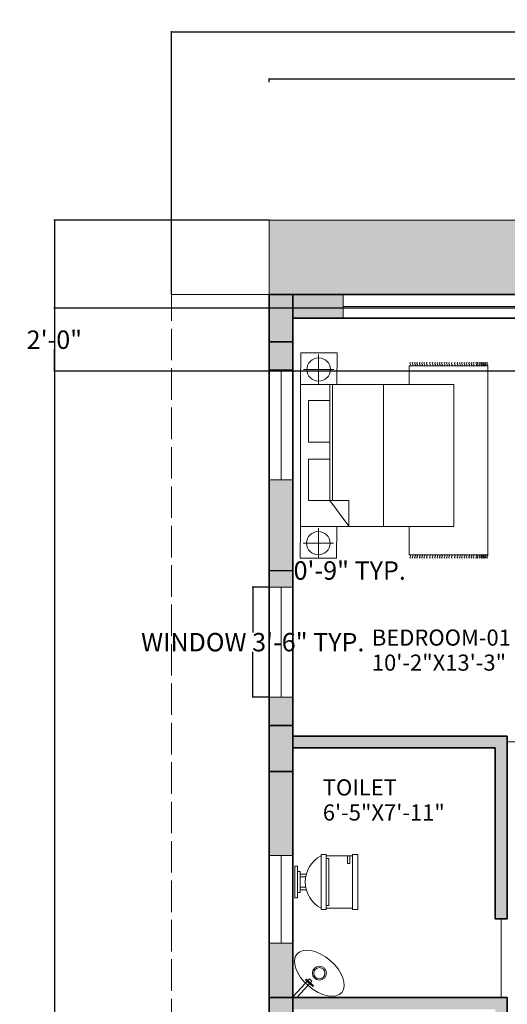
# Model space of a CAD drawing. Units: inches. Extents: x -17 to 892, y -721 to 172.
# Tile 4 of 11: x -12 to 174, y -209 to 166. Entities that reach past the tile are written whole.
import ezdxf

# ---------------------------------------------------------------- set-up
doc = ezdxf.new("R2010")
doc.units = ezdxf.units.IN
doc.header["$MEASUREMENT"] = 0
doc.linetypes.add('ACAD_ISO02W100', pattern=[15, 12, -3])
doc.layers.get('0').update_dxf_attribs({"color": 14})
for name, color, linetype, lineweight in [('A-ANNO-DIMS', 2, 'Continuous', 18), ('A-AREA-IDEN', 7, 'Continuous', 18), ('A-COLS', 252, 'Continuous', 35), ('A-FLOR-FIXT', 8, 'Continuous', 18), ('A-WALL-PATT', 14, 'Continuous', 13), ('C-PROP', 8, 'ACAD_ISO02W100', 18), ('C-ROAD', 8, 'Continuous', 18), ('doors', 4, 'Continuous', 18), ('furniture', 252, 'Continuous', 18), ('walls', 252, 'Continuous', 35), ('windows', 161, 'Continuous', 18)]:
    doc.layers.add(name, color=color, linetype=linetype, lineweight=lineweight)
doc.layers.add('A-COLS-PATT', color=254, linetype='Continuous', lineweight=13, true_color=0xd7ebd2)
doc.layers.add('C-ROAD-PATT', color=9, linetype='Continuous', lineweight=13, true_color=0xafd9aa)
doc.styles.get("Standard").update_dxf_attribs({"font": 'arial.ttf'})
doc.dimstyles.get("Standard").update_dxf_attribs({"dimtxt": 7, "dimasz": 0.18, "dimexe": 0.18, "dimexo": 0.0625, "dimgap": 0.09, "dimtad": 0, "dimtih": 1, "dimtoh": 1, "dimzin": 0, "dimdsep": 46, "dimlunit": 3, "dimtxsty": 'Standard', "dimcen": 0.09, "dimadec": 0, "dimazin": 0, "dimtfac": 1, "dimtofl": 0, "dimtmove": 0, "dimatfit": 3, "dimfxl": 1, "dimtolj": 1, "dimtzin": 0, "dimarcsym": 0})

# ---------------------------------------------------------------- blocks, each defined once
blk = doc.blocks.new('CARPET')
at = {"layer": 'furniture'}
for p, q in [((-51.53, -98.11), (-51.53, -55.12)), ((-51.53, -55.12), (-41.27, -55.12)), ((36, -55.12), (51.55, -55.12)), ((51.55, -55.12), (51.55, -98.11)), ((51.55, -98.11), (-51.53, -98.11))]:
    blk.add_line(p, q, dxfattribs=at)
for points, knots in [([(-53.37, -55.99), (-53.22, -55.8), (-52.9, -55.41), (-52.34, -55.8), (-51.89, -56.08), (-51.65, -55.91), (-51.53, -55.83)], [0, 0, 0, 0, 0.653278, 1.290138, 1.740457, 2.114451, 2.114451, 2.114451, 2.114451]), ([(-53.37, -57.26), (-53.22, -57.07), (-52.9, -56.67), (-52.34, -57.07), (-51.89, -57.35), (-51.65, -57.17), (-51.53, -57.1)], [0, 0, 0, 0, 0.653278, 1.290138, 1.740457, 2.114451, 2.114451, 2.114451, 2.114451]), ([(-53.37, -58.59), (-53.22, -58.4), (-52.9, -58.01), (-52.34, -58.4), (-51.89, -58.68), (-51.65, -58.5), (-51.53, -58.43)], [0, 0, 0, 0, 0.653278, 1.290138, 1.740457, 2.114451, 2.114451, 2.114451, 2.114451]), ([(53.37, -55.99), (53.22, -55.8), (52.9, -55.41), (52.34, -55.8), (51.89, -56.08), (51.65, -55.91), (51.53, -55.83)], [0, 0, 0, 0, 0.653278, 1.290138, 1.740457, 2.114451, 2.114451, 2.114451, 2.114451]), ([(53.37, -57.26), (53.22, -57.07), (52.9, -56.67), (52.34, -57.07), (51.89, -57.35), (51.65, -57.17), (51.53, -57.1)], [0, 0, 0, 0, 0.653278, 1.290138, 1.740457, 2.114451, 2.114451, 2.114451, 2.114451]), ([(53.37, -58.59), (53.22, -58.4), (52.9, -58.01), (52.34, -58.4), (51.89, -58.68), (51.65, -58.5), (51.53, -58.43)], [0, 0, 0, 0, 0.653278, 1.290138, 1.740457, 2.114451, 2.114451, 2.114451, 2.114451]), ([(-53.37, -59.78), (-53.22, -59.58), (-52.9, -59.19), (-52.34, -59.58), (-51.89, -59.86), (-51.65, -59.69), (-51.53, -59.61)], [0, 0, 0, 0, 0.653278, 1.290138, 1.740457, 2.114451, 2.114451, 2.114451, 2.114451]), ([(-53.37, -61.22), (-53.22, -61.02), (-52.9, -60.63), (-52.34, -61.02), (-51.89, -61.3), (-51.65, -61.13), (-51.53, -61.05)], [0, 0, 0, 0, 0.653278, 1.290138, 1.740457, 2.114451, 2.114451, 2.114451, 2.114451]), ([(-53.37, -62.44), (-53.22, -62.25), (-52.9, -61.86), (-52.34, -62.25), (-51.89, -62.53), (-51.65, -62.36), (-51.53, -62.28)], [0, 0, 0, 0, 0.653278, 1.290138, 1.740457, 2.114451, 2.114451, 2.114451, 2.114451]), ([(-53.37, -63.63), (-53.22, -63.43), (-52.9, -63.04), (-52.34, -63.43), (-51.89, -63.72), (-51.65, -63.54), (-51.53, -63.46)], [0, 0, 0, 0, 0.653278, 1.290138, 1.740457, 2.114451, 2.114451, 2.114451, 2.114451]), ([(53.37, -59.78), (53.22, -59.58), (52.9, -59.19), (52.34, -59.58), (51.89, -59.86), (51.65, -59.69), (51.53, -59.61)], [0, 0, 0, 0, 0.653278, 1.290138, 1.740457, 2.114451, 2.114451, 2.114451, 2.114451]), ([(53.37, -61.22), (53.22, -61.02), (52.9, -60.63), (52.34, -61.02), (51.89, -61.3), (51.65, -61.13), (51.53, -61.05)], [0, 0, 0, 0, 0.653278, 1.290138, 1.740457, 2.114451, 2.114451, 2.114451, 2.114451]), ([(53.37, -62.44), (53.22, -62.25), (52.9, -61.86), (52.34, -62.25), (51.89, -62.53), (51.65, -62.36), (51.53, -62.28)], [0, 0, 0, 0, 0.653278, 1.290138, 1.740457, 2.114451, 2.114451, 2.114451, 2.114451]), ([(53.37, -63.63), (53.22, -63.43), (52.9, -63.04), (52.34, -63.43), (51.89, -63.72), (51.65, -63.54), (51.53, -63.46)], [0, 0, 0, 0, 0.653278, 1.290138, 1.740457, 2.114451, 2.114451, 2.114451, 2.114451]), ([(-53.37, -65.07), (-53.22, -64.87), (-52.9, -64.48), (-52.34, -64.87), (-51.89, -65.15), (-51.65, -64.98), (-51.53, -64.9)], [0, 0, 0, 0, 0.653278, 1.290138, 1.740457, 2.114451, 2.114451, 2.114451, 2.114451]), ([(-53.37, -66.76), (-53.22, -66.56), (-52.9, -66.17), (-52.34, -66.56), (-51.89, -66.84), (-51.65, -66.67), (-51.53, -66.59)], [0, 0, 0, 0, 0.653278, 1.290138, 1.740457, 2.114451, 2.114451, 2.114451, 2.114451]), ([(-53.37, -68.2), (-53.22, -68), (-52.9, -67.61), (-52.34, -68), (-51.89, -68.28), (-51.65, -68.11), (-51.53, -68.03)], [0, 0, 0, 0, 0.653278, 1.290138, 1.740457, 2.114451, 2.114451, 2.114451, 2.114451]), ([(-53.37, -69.53), (-53.22, -69.33), (-52.9, -68.94), (-52.34, -69.33), (-51.89, -69.61), (-51.65, -69.44), (-51.53, -69.36)], [0, 0, 0, 0, 0.653278, 1.290138, 1.740457, 2.114451, 2.114451, 2.114451, 2.114451]), ([(53.37, -65.07), (53.22, -64.87), (52.9, -64.48), (52.34, -64.87), (51.89, -65.15), (51.65, -64.98), (51.53, -64.9)], [0, 0, 0, 0, 0.653278, 1.290138, 1.740457, 2.114451, 2.114451, 2.114451, 2.114451]), ([(53.37, -66.76), (53.22, -66.56), (52.9, -66.17), (52.34, -66.56), (51.89, -66.84), (51.65, -66.67), (51.53, -66.59)], [0, 0, 0, 0, 0.653278, 1.290138, 1.740457, 2.114451, 2.114451, 2.114451, 2.114451]), ([(53.37, -68.2), (53.22, -68), (52.9, -67.61), (52.34, -68), (51.89, -68.28), (51.65, -68.11), (51.53, -68.03)], [0, 0, 0, 0, 0.653278, 1.290138, 1.740457, 2.114451, 2.114451, 2.114451, 2.114451]), ([(53.37, -69.53), (53.22, -69.33), (52.9, -68.94), (52.34, -69.33), (51.89, -69.61), (51.65, -69.44), (51.53, -69.36)], [0, 0, 0, 0, 0.653278, 1.290138, 1.740457, 2.114451, 2.114451, 2.114451, 2.114451]), ([(-53.37, -70.79), (-53.22, -70.6), (-52.9, -70.21), (-52.34, -70.6), (-51.89, -70.88), (-51.65, -70.7), (-51.53, -70.63)], [0, 0, 0, 0, 0.653278, 1.290138, 1.740457, 2.114451, 2.114451, 2.114451, 2.114451]), ([(-53.37, -72.12), (-53.22, -71.93), (-52.9, -71.54), (-52.34, -71.93), (-51.89, -72.21), (-51.65, -72.04), (-51.53, -71.96)], [0, 0, 0, 0, 0.653278, 1.290138, 1.740457, 2.114451, 2.114451, 2.114451, 2.114451]), ([(-53.37, -73.31), (-53.22, -73.11), (-52.9, -72.72), (-52.34, -73.11), (-51.89, -73.4), (-51.65, -73.22), (-51.53, -73.14)], [0, 0, 0, 0, 0.653278, 1.290138, 1.740457, 2.114451, 2.114451, 2.114451, 2.114451]), ([(-53.37, -74.75), (-53.22, -74.55), (-52.9, -74.16), (-52.34, -74.55), (-51.89, -74.83), (-51.65, -74.66), (-51.53, -74.58)], [0, 0, 0, 0, 0.653278, 1.290138, 1.740457, 2.114451, 2.114451, 2.114451, 2.114451]), ([(53.37, -70.79), (53.22, -70.6), (52.9, -70.21), (52.34, -70.6), (51.89, -70.88), (51.65, -70.7), (51.53, -70.63)], [0, 0, 0, 0, 0.653278, 1.290138, 1.740457, 2.114451, 2.114451, 2.114451, 2.114451]), ([(53.37, -72.12), (53.22, -71.93), (52.9, -71.54), (52.34, -71.93), (51.89, -72.21), (51.65, -72.04), (51.53, -71.96)], [0, 0, 0, 0, 0.653278, 1.290138, 1.740457, 2.114451, 2.114451, 2.114451, 2.114451]), ([(53.37, -73.31), (53.22, -73.11), (52.9, -72.72), (52.34, -73.11), (51.89, -73.4), (51.65, -73.22), (51.53, -73.14)], [0, 0, 0, 0, 0.653278, 1.290138, 1.740457, 2.114451, 2.114451, 2.114451, 2.114451]), ([(53.37, -74.75), (53.22, -74.55), (52.9, -74.16), (52.34, -74.55), (51.89, -74.83), (51.65, -74.66), (51.53, -74.58)], [0, 0, 0, 0, 0.653278, 1.290138, 1.740457, 2.114451, 2.114451, 2.114451, 2.114451]), ([(-53.37, -75.98), (-53.22, -75.78), (-52.9, -75.39), (-52.34, -75.78), (-51.89, -76.06), (-51.65, -75.89), (-51.53, -75.81)], [0, 0, 0, 0, 0.653278, 1.290138, 1.740457, 2.114451, 2.114451, 2.114451, 2.114451]), ([(-53.37, -77.16), (-53.22, -76.96), (-52.9, -76.57), (-52.34, -76.96), (-51.89, -77.25), (-51.65, -77.07), (-51.53, -76.99)], [0, 0, 0, 0, 0.653278, 1.290138, 1.740457, 2.114451, 2.114451, 2.114451, 2.114451]), ([(-53.37, -78.6), (-53.22, -78.4), (-52.9, -78.01), (-52.34, -78.4), (-51.89, -78.68), (-51.65, -78.51), (-51.53, -78.43)], [0, 0, 0, 0, 0.653278, 1.290138, 1.740457, 2.114451, 2.114451, 2.114451, 2.114451]), ([(-53.37, -80.29), (-53.22, -80.09), (-52.9, -79.7), (-52.34, -80.09), (-51.89, -80.37), (-51.65, -80.2), (-51.53, -80.12)], [0, 0, 0, 0, 0.653278, 1.290138, 1.740457, 2.114451, 2.114451, 2.114451, 2.114451]), ([(53.37, -75.98), (53.22, -75.78), (52.9, -75.39), (52.34, -75.78), (51.89, -76.06), (51.65, -75.89), (51.53, -75.81)], [0, 0, 0, 0, 0.653278, 1.290138, 1.740457, 2.114451, 2.114451, 2.114451, 2.114451]), ([(53.37, -77.16), (53.22, -76.96), (52.9, -76.57), (52.34, -76.96), (51.89, -77.25), (51.65, -77.07), (51.53, -76.99)], [0, 0, 0, 0, 0.653278, 1.290138, 1.740457, 2.114451, 2.114451, 2.114451, 2.114451]), ([(53.37, -78.6), (53.22, -78.4), (52.9, -78.01), (52.34, -78.4), (51.89, -78.68), (51.65, -78.51), (51.53, -78.43)], [0, 0, 0, 0, 0.653278, 1.290138, 1.740457, 2.114451, 2.114451, 2.114451, 2.114451]), ([(53.37, -80.29), (53.22, -80.09), (52.9, -79.7), (52.34, -80.09), (51.89, -80.37), (51.65, -80.2), (51.53, -80.12)], [0, 0, 0, 0, 0.653278, 1.290138, 1.740457, 2.114451, 2.114451, 2.114451, 2.114451]), ([(-53.37, -81.73), (-53.22, -81.53), (-52.9, -81.14), (-52.34, -81.53), (-51.89, -81.81), (-51.65, -81.64), (-51.53, -81.56)], [0, 0, 0, 0, 0.653278, 1.290138, 1.740457, 2.114451, 2.114451, 2.114451, 2.114451]), ([(-53.37, -83.06), (-53.22, -82.86), (-52.9, -82.47), (-52.34, -82.86), (-51.89, -83.14), (-51.65, -82.97), (-51.53, -82.89)], [0, 0, 0, 0, 0.653278, 1.290138, 1.740457, 2.114451, 2.114451, 2.114451, 2.114451]), ([(-53.37, -84.18), (-53.22, -83.99), (-52.9, -83.6), (-52.34, -83.99), (-51.89, -84.27), (-51.65, -84.09), (-51.53, -84.02)], [0, 0, 0, 0, 0.653278, 1.290138, 1.740457, 2.114451, 2.114451, 2.114451, 2.114451]), ([(-53.37, -85.51), (-53.22, -85.32), (-52.9, -84.93), (-52.34, -85.32), (-51.89, -85.6), (-51.65, -85.42), (-51.53, -85.35)], [0, 0, 0, 0, 0.653278, 1.290138, 1.740457, 2.114451, 2.114451, 2.114451, 2.114451]), ([(53.37, -81.73), (53.22, -81.53), (52.9, -81.14), (52.34, -81.53), (51.89, -81.81), (51.65, -81.64), (51.53, -81.56)], [0, 0, 0, 0, 0.653278, 1.290138, 1.740457, 2.114451, 2.114451, 2.114451, 2.114451]), ([(53.37, -83.06), (53.22, -82.86), (52.9, -82.47), (52.34, -82.86), (51.89, -83.14), (51.65, -82.97), (51.53, -82.89)], [0, 0, 0, 0, 0.653278, 1.290138, 1.740457, 2.114451, 2.114451, 2.114451, 2.114451]), ([(53.37, -84.18), (53.22, -83.99), (52.9, -83.6), (52.34, -83.99), (51.89, -84.27), (51.65, -84.09), (51.53, -84.02)], [0, 0, 0, 0, 0.653278, 1.290138, 1.740457, 2.114451, 2.114451, 2.114451, 2.114451]), ([(53.37, -85.51), (53.22, -85.32), (52.9, -84.93), (52.34, -85.32), (51.89, -85.6), (51.65, -85.42), (51.53, -85.35)], [0, 0, 0, 0, 0.653278, 1.290138, 1.740457, 2.114451, 2.114451, 2.114451, 2.114451]), ([(-53.37, -86.7), (-53.22, -86.5), (-52.9, -86.11), (-52.34, -86.5), (-51.89, -86.78), (-51.65, -86.61), (-51.53, -86.53)], [0, 0, 0, 0, 0.653278, 1.290138, 1.740457, 2.114451, 2.114451, 2.114451, 2.114451]), ([(-53.37, -88.14), (-53.22, -87.94), (-52.9, -87.55), (-52.34, -87.94), (-51.89, -88.22), (-51.65, -88.05), (-51.53, -87.97)], [0, 0, 0, 0, 0.653278, 1.290138, 1.740457, 2.114451, 2.114451, 2.114451, 2.114451]), ([(-53.37, -89.36), (-53.22, -89.17), (-52.9, -88.78), (-52.34, -89.17), (-51.89, -89.45), (-51.65, -89.28), (-51.53, -89.2)], [0, 0, 0, 0, 0.653278, 1.290138, 1.740457, 2.114451, 2.114451, 2.114451, 2.114451]), ([(-53.37, -90.55), (-53.22, -90.35), (-52.9, -89.96), (-52.34, -90.35), (-51.89, -90.64), (-51.65, -90.46), (-51.53, -90.38)], [0, 0, 0, 0, 0.653278, 1.290138, 1.740457, 2.114451, 2.114451, 2.114451, 2.114451]), ([(53.37, -86.7), (53.22, -86.5), (52.9, -86.11), (52.34, -86.5), (51.89, -86.78), (51.65, -86.61), (51.53, -86.53)], [0, 0, 0, 0, 0.653278, 1.290138, 1.740457, 2.114451, 2.114451, 2.114451, 2.114451]), ([(53.37, -88.14), (53.22, -87.94), (52.9, -87.55), (52.34, -87.94), (51.89, -88.22), (51.65, -88.05), (51.53, -87.97)], [0, 0, 0, 0, 0.653278, 1.290138, 1.740457, 2.114451, 2.114451, 2.114451, 2.114451]), ([(53.37, -89.36), (53.22, -89.17), (52.9, -88.78), (52.34, -89.17), (51.89, -89.45), (51.65, -89.28), (51.53, -89.2)], [0, 0, 0, 0, 0.653278, 1.290138, 1.740457, 2.114451, 2.114451, 2.114451, 2.114451]), ([(53.37, -90.55), (53.22, -90.35), (52.9, -89.96), (52.34, -90.35), (51.9, -90.63), (51.66, -90.47), (51.55, -90.4)], [0, 0, 0, 0, 0.653278, 1.290138, 1.740457, 2.0926, 2.0926, 2.0926, 2.0926]), ([(-53.37, -91.99), (-53.22, -91.79), (-52.9, -91.4), (-52.34, -91.79), (-51.89, -92.07), (-51.65, -91.9), (-51.53, -91.82)], [0, 0, 0, 0, 0.653278, 1.290138, 1.740457, 2.114451, 2.114451, 2.114451, 2.114451]), ([(-53.37, -92.69), (-53.22, -92.48), (-52.9, -92.08), (-52.35, -92.49), (-51.89, -92.77), (-51.65, -92.6), (-51.53, -92.52)], [0, 0, 0, 0, 0.663904, 1.307406, 1.757725, 2.131719, 2.131719, 2.131719, 2.131719]), ([(-53.37, -93.61), (-53.22, -93.42), (-52.9, -93.03), (-52.34, -93.42), (-51.89, -93.7), (-51.65, -93.52), (-51.53, -93.45)], [0, 0, 0, 0, 0.653278, 1.290138, 1.740457, 2.114451, 2.114451, 2.114451, 2.114451]), ([(-53.37, -94.55), (-53.22, -94.35), (-52.9, -93.96), (-52.34, -94.35), (-51.89, -94.63), (-51.65, -94.46), (-51.53, -94.38)], [0, 0, 0, 0, 0.653278, 1.290138, 1.740457, 2.114451, 2.114451, 2.114451, 2.114451]), ([(-53.37, -95.05), (-53.22, -94.85), (-52.9, -94.46), (-52.34, -94.85), (-51.89, -95.14), (-51.65, -94.96), (-51.53, -94.88)], [0, 0, 0, 0, 0.653278, 1.290138, 1.740457, 2.114451, 2.114451, 2.114451, 2.114451]), ([(-53.37, -95.73), (-53.22, -95.54), (-52.9, -95.15), (-52.34, -95.54), (-51.89, -95.82), (-51.65, -95.65), (-51.53, -95.57)], [0, 0, 0, 0, 0.653278, 1.290138, 1.740457, 2.114451, 2.114451, 2.114451, 2.114451]), ([(-53.37, -96.38), (-53.22, -96.18), (-52.9, -95.79), (-52.34, -96.18), (-51.89, -96.47), (-51.65, -96.29), (-51.53, -96.21)], [0, 0, 0, 0, 0.653278, 1.290138, 1.740457, 2.114451, 2.114451, 2.114451, 2.114451]), ([(53.37, -95.78), (53.22, -95.58), (52.9, -95.19), (52.34, -95.58), (51.89, -95.86), (51.65, -95.69), (51.53, -95.61)], [0, 0, 0, 0, 0.653278, 1.290138, 1.740457, 2.114451, 2.114451, 2.114451, 2.114451]), ([(53.37, -96.43), (53.22, -96.23), (52.9, -95.84), (52.34, -96.23), (51.89, -96.51), (51.65, -96.34), (51.53, -96.26)], [0, 0, 0, 0, 0.653278, 1.290138, 1.740457, 2.114451, 2.114451, 2.114451, 2.114451]), ([(53.37, -91.99), (53.22, -91.79), (52.9, -91.4), (52.34, -91.79), (51.9, -92.07), (51.66, -91.91), (51.55, -91.83)], [0, 0, 0, 0, 0.653278, 1.290138, 1.740457, 2.0926, 2.0926, 2.0926, 2.0926]), ([(53.37, -92.69), (53.22, -92.49), (52.9, -92.09), (52.34, -92.49), (51.9, -92.77), (51.66, -92.61), (51.55, -92.53)], [0, 0, 0, 0, 0.656792, 1.295826, 1.746145, 2.098292, 2.098292, 2.098292, 2.098292]), ([(53.37, -93.66), (53.22, -93.46), (52.9, -93.07), (52.34, -93.46), (51.9, -93.74), (51.66, -93.58), (51.55, -93.5)], [0, 0, 0, 0, 0.653278, 1.290138, 1.740457, 2.0926, 2.0926, 2.0926, 2.0926]), ([(53.37, -94.59), (53.22, -94.4), (52.9, -94.01), (52.34, -94.4), (51.9, -94.68), (51.66, -94.51), (51.55, -94.44)], [0, 0, 0, 0, 0.653278, 1.290138, 1.740457, 2.0926, 2.0926, 2.0926, 2.0926]), ([(53.37, -95.1), (53.22, -94.9), (52.9, -94.51), (52.34, -94.9), (51.9, -95.18), (51.66, -95.02), (51.55, -94.94)], [0, 0, 0, 0, 0.653278, 1.290138, 1.740457, 2.0926, 2.0926, 2.0926, 2.0926]), ([(-53.37, -97.17), (-53.22, -96.98), (-52.9, -96.59), (-52.34, -96.98), (-51.89, -97.26), (-51.65, -97.08), (-51.53, -97.01)], [0, 0, 0, 0, 0.653278, 1.290138, 1.740457, 2.114451, 2.114451, 2.114451, 2.114451]), ([(-53.37, -97.99), (-53.22, -97.79), (-52.9, -97.4), (-52.34, -97.79), (-51.89, -98.08), (-51.65, -97.9), (-51.53, -97.82)], [0, 0, 0, 0, 0.653278, 1.290138, 1.740457, 2.114451, 2.114451, 2.114451, 2.114451]), ([(53.37, -97.22), (53.22, -97.02), (52.9, -96.63), (52.34, -97.02), (51.89, -97.3), (51.65, -97.13), (51.53, -97.05)], [0, 0, 0, 0, 0.653278, 1.290138, 1.740457, 2.114451, 2.114451, 2.114451, 2.114451]), ([(53.37, -97.99), (53.22, -97.79), (52.9, -97.4), (52.34, -97.79), (51.89, -98.08), (51.65, -97.9), (51.53, -97.82)], [0, 0, 0, 0, 0.653278, 1.290138, 1.740457, 2.114451, 2.114451, 2.114451, 2.114451])]:
    blk.add_open_spline(points, degree=3, knots=knots, dxfattribs=at)
blk = doc.blocks.new('A$C58D270C6')
at = {"layer": 'furniture'}
for p, q in [((9.09, 124.13), (9.09, 108.87)), ((1.46, 116.5), (16.73, 116.5)), ((14.97, 94.84), (24.62, 107.92)), ((24.62, 94.93), (24.62, 107.92)), ((42.08, 108), (42.08, 36)), ((14.97, 94.93), (24.62, 94.93)), ((14.97, 94.84), (14.97, 36)), ((16.22, 94.93), (16.22, 36)), ((9.25, 36), (9.25, 20.74)), ((1.62, 28.37), (16.88, 28.37))]:
    blk.add_line(p, q, dxfattribs=at)
for points in [[(18.5, 108), (18.34, 124.13), (-0.16, 124.13), (0, 108)], [(0, 108), (77.91, 108), (77.91, 36), (0, 36)], [(4.09, 94.93), (14.97, 94.93), (14.97, 73.83), (4.09, 73.83)], [(4.09, 65.23), (14.97, 65.23), (14.97, 44.13), (4.09, 44.13)], [(18.65, 19.87), (18.5, 36), (0, 36), (0.16, 19.87)]]:
    blk.add_lwpolyline(points, close=True, dxfattribs=at)
for centre in [(9.09, 116.5), (9.25, 28.37)]:
    blk.add_circle(centre, 5.95, dxfattribs=at)
at = {"layer": 'furniture', "xscale": 0.9312884925094044, "yscale": 0.9312884925094044, "zscale": 0.9312884925094044, "rotation": 90}
blk.add_blockref('CARPET', (3.79, 74.47), dxfattribs=at)
blk = doc.blocks.new('*U12')
for p, q in [((-10, 22), (-10, 12)), ((-10, 21), (-7, 21)), ((-7, 20), (-10, 20)), ((-7, 21), (-7, 20)), ((10, 12), (10, 22)), ((10.5, 12), (-10.5, 12)), ((-10.5, 10), (-10.5, 12)), ((9, 13), (-9, 13)), ((-9, 13), (-9, 12)), ((9, 12), (9, 13)), ((10.5, 12), (10.5, 10)), ((10.5, 10), (-10.5, 10)), ((-3, 4.4065), (-3, 2)), ((-2, 2), (-2, 4.1658)), ((2, 4.1658), (2, 2)), ((3, 2), (3, 4.4065)), ((4, 2), (-4, 2)), ((-4, 2), (-4, 1)), ((4, 1), (4, 2))]:
    blk.add_line(p, q)
for points in [[(10.5, 22), (10.5, 24), (-10.5, 24), (-10.5, 22)], [(6, 0), (6, 1), (-6, 1), (-6, 0)]]:
    blk.add_lwpolyline(points, close=True)
blk.add_arc((0, 15.3333), 11.3333, 208.0725, 331.9275)
blk = doc.blocks.new('*D15')
at = {"layer": 'A-ANNO-DIMS', "color": 0, "lineweight": -2, "transparency": 16777216}
for p, q in [((83.08, 142.49), (83.08, 143.87)), ((83.26, 143.69), (208.99, 143.69)), ((346.9, 143.69), (221.17, 143.69)), ((347.08, 142.49), (347.08, 143.87))]:
    blk.add_line(p, q, dxfattribs=at)
at = {"layer": 'A-ANNO-DIMS', "color": 0, "lineweight": 100, "transparency": 16777216}
for points in [[(83.26, 143.72), (83.26, 143.66), (83.08, 143.69)], [(346.9, 143.72), (346.9, 143.66), (347.08, 143.69)]]:
    blk.add_solid(points, dxfattribs=at)
at = {"layer": 'Defpoints', "color": 0, "lineweight": 100, "transparency": 16777216}
for p in [(83.08, 142.43), (347.08, 143.69), (347.08, 142.43)]:
    blk.add_point(p, dxfattribs=at)
at = {"layer": 'A-ANNO-DIMS', "color": 0, "transparency": 16777216, "insert": (215.08, 143.69), "char_height": 7, "attachment_point": 5}
blk.add_mtext("\\A1;22'", dxfattribs=at)
blk = doc.blocks.new('WIN-42-FRAMED')
for p, q in [((0, 41.96), (9, 41.96)), ((0, 0), (0, 41.96)), ((0, 41.96), (4.5, 41.96)), ((4.5, 41.96), (4.5, 0)), ((9, 41.96), (9, 0)), ((9, 0), (0, 0))]:
    blk.add_line(p, q)
blk = doc.blocks.new('WIN-68-INSET')
for p, q in [((0, 9), (0, 0)), ((0, 9), (0, 4.5)), ((67.89, 0), (67.89, 9)), ((0, 4.5), (67.89, 4.5))]:
    blk.add_line(p, q)
blk = doc.blocks.new('*D38')
at = {"layer": 'A-ANNO-DIMS', "color": 0, "lineweight": -2, "transparency": 16777216}
for p, q in [((83.02, -49.69), (76.61, -49.69)), ((76.79, -49.87), (76.79, -66.96)), ((76.79, -91.47), (76.79, -74.38)), ((83.02, -91.65), (76.61, -91.65))]:
    blk.add_line(p, q, dxfattribs=at)
at = {"layer": 'A-ANNO-DIMS', "color": 0, "lineweight": 100, "transparency": 16777216}
for points in [[(76.76, -49.87), (76.82, -49.87), (76.79, -49.69)], [(76.76, -91.47), (76.82, -91.47), (76.79, -91.65)]]:
    blk.add_solid(points, dxfattribs=at)
at = {"layer": 'Defpoints', "color": 0, "lineweight": 100, "transparency": 16777216}
for p in [(76.79, -49.69), (83.08, -49.69), (83.08, -91.65)]:
    blk.add_point(p, dxfattribs=at)
at = {"layer": 'A-ANNO-DIMS', "color": 0, "transparency": 16777216, "insert": (76.79, -70.67), "char_height": 7, "attachment_point": 5}
blk.add_mtext('\\A1;WINDOW 3\'-6" TYP.', dxfattribs=at)
blk = doc.blocks.new('*D39')
at = {"layer": 'A-ANNO-DIMS', "color": 0, "lineweight": -2, "transparency": 16777216}
for p, q in [((83.08, -49.63), (83.08, -43.22)), ((83.26, -43.4), (91.9, -43.4)), ((92.08, -49.63), (92.08, -43.22)), ((92.08, -43.4), (92.26, -43.4))]:
    blk.add_line(p, q, dxfattribs=at)
at = {"layer": 'A-ANNO-DIMS', "color": 0, "lineweight": 100, "transparency": 16777216}
for points in [[(83.26, -43.37), (83.26, -43.43), (83.08, -43.4)], [(91.9, -43.37), (91.9, -43.43), (92.08, -43.4)]]:
    blk.add_solid(points, dxfattribs=at)
at = {"layer": 'Defpoints', "color": 0, "lineweight": 100, "transparency": 16777216}
for p in [(92.08, -43.4), (83.08, -49.69), (92.08, -49.69)]:
    blk.add_point(p, dxfattribs=at)
at = {"layer": 'A-ANNO-DIMS', "color": 0, "transparency": 16777216, "insert": (113.69, -43.4), "char_height": 7, "attachment_point": 5}
blk.add_mtext('\\A1;0\'-9" TYP.', dxfattribs=at)
blk = doc.blocks.new('*D56')
at = {"layer": 'A-ANNO-DIMS', "color": 0, "lineweight": -2, "transparency": 16777216}
for p, q in [((45.89, 61.67), (45.89, 161.84)), ((46.07, 161.66), (184.32, 161.66)), ((346.9, 161.66), (208.66, 161.66)), ((347.08, 89.96), (347.08, 161.84))]:
    blk.add_line(p, q, dxfattribs=at)
at = {"layer": 'A-ANNO-DIMS', "color": 0, "lineweight": 100, "transparency": 16777216}
for points in [[(46.07, 161.69), (46.07, 161.63), (45.89, 161.66)], [(346.9, 161.69), (346.9, 161.63), (347.08, 161.66)]]:
    blk.add_solid(points, dxfattribs=at)
at = {"layer": 'Defpoints', "color": 0, "lineweight": 100, "transparency": 16777216}
for p in [(45.89, 161.66), (347.08, 89.9), (45.89, 61.61)]:
    blk.add_point(p, dxfattribs=at)
at = {"layer": 'A-ANNO-DIMS', "color": 0, "transparency": 16777216, "insert": (196.49, 161.66), "char_height": 7, "attachment_point": 5}
blk.add_mtext('\\A1;25\'-1"', dxfattribs=at)
blk = doc.blocks.new('*D57')
at = {"layer": 'A-ANNO-DIMS', "color": 0, "lineweight": -2, "transparency": 16777216}
for p, q in [((83.02, 89.9), (1.11, 89.9)), ((1.29, 89.72), (1.29, -281.05)), ((1.29, -659.16), (1.29, -288.38)), ((83.02, -659.34), (1.11, -659.34))]:
    blk.add_line(p, q, dxfattribs=at)
at = {"layer": 'A-ANNO-DIMS', "color": 0, "lineweight": 100, "transparency": 16777216}
for points in [[(1.26, 89.72), (1.32, 89.72), (1.29, 89.9)], [(1.26, -659.16), (1.32, -659.16), (1.29, -659.34)]]:
    blk.add_solid(points, dxfattribs=at)
at = {"layer": 'Defpoints', "color": 0, "lineweight": 100, "transparency": 16777216}
for p in [(1.29, 89.9), (83.08, 89.9), (83.08, -659.34)]:
    blk.add_point(p, dxfattribs=at)
at = {"layer": 'A-ANNO-DIMS', "color": 0, "transparency": 16777216, "insert": (1.29, -284.72), "char_height": 7, "attachment_point": 5}
blk.add_mtext('\\A1;62\'-5"', dxfattribs=at)
blk = doc.blocks.new('*D68')
at = {"layer": 'A-ANNO-DIMS', "color": 0, "lineweight": -2, "transparency": 16777216}
for p, q in [((738.65, 56.46), (1.11, 56.46)), ((1.29, 56.28), (1.29, 48.13)), ((1.29, 32.64), (1.29, 40.8)), ((737.65, 32.46), (1.11, 32.46))]:
    blk.add_line(p, q, dxfattribs=at)
at = {"layer": 'A-ANNO-DIMS', "color": 0, "lineweight": 100, "transparency": 16777216}
for points in [[(1.26, 56.28), (1.32, 56.28), (1.29, 56.46)], [(1.26, 32.64), (1.32, 32.64), (1.29, 32.46)]]:
    blk.add_solid(points, dxfattribs=at)
at = {"layer": 'Defpoints', "color": 0, "lineweight": 100, "transparency": 16777216}
for p in [(738.71, 56.46), (1.29, 32.46), (737.71, 32.46)]:
    blk.add_point(p, dxfattribs=at)
at = {"layer": 'A-ANNO-DIMS', "color": 0, "transparency": 16777216, "insert": (1.29, 44.46), "char_height": 7, "attachment_point": 5}
blk.add_mtext('\\A1;2\'-0"', dxfattribs=at)

msp = doc.modelspace()

# ---------------------------------------------------------------- hatches: boundary and pattern name
at = {"layer": 'A-COLS-PATT'}
h = msp.add_hatch(color=256, dxfattribs=at)
h.dxf.hatch_style = 1
h.paths.add_polyline_path([(92.084, 61.611), (83.084, 61.611), (83.084, 43.692), (92.084, 43.692)])
h.paths.add_polyline_path([(347.084, 61.611), (338.084, 61.611), (338.084, 43.692), (347.084, 43.692)])
h.paths.add_polyline_path([(222.053, 61.611), (209.95, 61.611), (209.95, 52.611), (222.053, 52.611)])
h.paths.add_polyline_path([(284.798, 61.611), (274.584, 61.611), (274.584, 52.611), (284.798, 52.611)])
h.paths.add_polyline_path([(223.084, -106.389), (214.084, -106.389), (214.084, -119.959), (223.084, -119.959)])
h.paths.add_polyline_path([(347.084, -148.653), (338.084, -148.653), (338.084, -172.24), (347.084, -172.24)])
h.paths.add_polyline_path([(92.084, -102.402), (83.084, -102.402), (83.084, -119.959), (92.084, -119.959)])
h.paths.add_polyline_path([(92.084, -205.889), (83.084, -205.889), (83.084, -216.319), (92.084, -216.319)])
h.paths.add_polyline_path([(347.084, -349.073), (338.084, -349.073), (338.084, -372.66), (347.084, -372.66)])
h.paths.add_polyline_path([(347.084, -610.134), (338.084, -610.134), (338.084, -614.389), (338.084, -623.342), (347.084, -623.342)])
h.paths.add_polyline_path([(221.166, -610.357), (214.084, -610.357), (214.084, -623.389), (219.084, -623.389), (221.166, -623.389), (221.166, -621.723)])
h.paths.add_polyline_path([(90.166, -610.357), (83.084, -610.357), (83.084, -623.389), (90.166, -623.389)])
h.paths.add_polyline_path([(223.084, -401.64), (214.084, -401.64), (214.084, -410.389), (223.084, -410.389)])
h.paths.add_polyline_path([(223.084, -356.889), (214.084, -356.889), (214.084, -369.273), (223.084, -369.273)])
h.paths.add_polyline_path([(92.084, -398.492), (83.084, -398.492), (83.084, -410.389), (92.084, -410.389)])
h.paths.add_polyline_path([(92.084, -348.918), (83.084, -348.918), (83.084, -360.706), (92.084, -360.706)])
h = msp.add_hatch(color=256, dxfattribs=at)
h.dxf.hatch_style = 1
h.paths.add_polyline_path([(92.084, -102.402), (83.084, -102.402), (83.084, -119.959), (92.084, -119.959)])
h.paths.add_polyline_path([(669.576, 61.611), (664.576, 61.611), (664.576, 57.111), (669.576, 57.111)])
h.paths.add_polyline_path([(676.541, 61.611), (669.576, 61.611), (669.576, 57.111), (676.541, 57.111)])
h.paths.add_polyline_path([(669.576, 57.111), (664.576, 57.111), (664.576, 53.097), (669.576, 53.097)])
h.paths.add_polyline_path([(676.541, 57.111), (669.576, 57.111), (669.576, 53.097), (676.541, 53.097)])
h.paths.add_polyline_path([(735.904, 61.611), (729.183, 61.611), (729.183, 57.111), (735.904, 57.111)])
h.paths.add_polyline_path([(735.904, 57.111), (729.183, 57.111), (729.183, 53.097), (735.904, 53.097)])
at = {"layer": 'A-WALL-PATT'}
h = msp.add_hatch(color=256, dxfattribs=at)
h.dxf.hatch_style = 1
h.paths.add_polyline_path([(111.26, 61.611), (92.084, 61.611), (92.084, 52.611), (111.26, 52.611)])
h.paths.add_polyline_path([(209.95, 61.611), (179.154, 61.611), (179.154, 52.611), (209.95, 52.611)])
h.paths.add_polyline_path([(338.084, 61.611), (284.798, 61.611), (284.798, 52.611), (338.084, 52.611)])
h.paths.add_polyline_path([(279.084, 23.861), (274.584, 23.861), (274.584, -0.389), (279.084, -0.389)])
h.paths.add_polyline_path([(279.084, 52.611), (274.584, 52.611), (274.584, 46.881), (276.834, 46.881), (279.084, 46.881)])
h.paths.add_polyline_path([(279.084, -0.389), (274.584, -0.389), (274.584, -4.889), (279.084, -4.889)])
h.paths.add_polyline_path([(304.22, -0.389), (279.084, -0.389), (279.084, -4.889), (304.22, -4.889)])
h.paths.add_polyline_path([(347.084, 43.692), (338.084, 43.692), (338.084, -148.653), (347.084, -148.653)])
h.paths.add_polyline_path([(338.084, -154.889), (264.103, -154.889), (264.103, -163.889), (338.084, -163.889)])
h.paths.add_polyline_path([(223.084, -119.959), (214.084, -119.959), (214.084, -163.889), (223.084, -163.889)])
h.paths.add_polyline_path([(218.584, 52.611), (214.084, 52.611), (214.084, -106.389), (218.584, -106.389)])
h.paths.add_polyline_path([(92.084, -8.943), (83.084, -8.943), (83.084, -49.69), (87.584, -49.69), (92.084, -49.69)])
h.paths.add_polyline_path([(92.084, 43.692), (83.084, 43.692), (83.084, 33.018), (87.584, 33.018), (92.084, 33.018)])
h.paths.add_polyline_path([(92.084, -91.651), (83.084, -91.651), (83.084, -102.402), (92.084, -102.402)])
h.paths.add_polyline_path([(92.084, -119.959), (83.084, -119.959), (83.084, -151.855), (87.584, -151.855), (92.084, -151.855)])
h.paths.add_polyline_path([(173.584, -108.639), (173.584, -106.389), (173.084, -106.389), (92.084, -106.389), (92.084, -110.889), (169.084, -110.889), (169.084, -176.029), (173.584, -176.029)])
h.paths.add_polyline_path([(92.084, -185.221), (83.084, -185.221), (83.084, -205.889), (92.084, -205.889)])
h.paths.add_polyline_path([(92.084, -216.319), (83.084, -216.319), (83.084, -259.015), (87.584, -259.015), (92.084, -259.015)])
h.paths.add_polyline_path([(173.584, -205.889), (92.084, -205.889), (92.084, -210.389), (169.084, -210.389), (169.084, -236.193), (173.584, -236.193)])
h.paths.add_polyline_path([(92.084, -300.976), (83.084, -300.976), (83.084, -348.918), (92.084, -348.918)])
h.paths.add_polyline_path([(87.584, -410.389), (83.084, -410.389), (83.084, -610.357), (87.584, -610.357)])
h.paths.add_polyline_path([(115.523, -614.389), (90.166, -614.389), (90.166, -623.389), (115.523, -623.389)])
h.paths.add_polyline_path([(214.084, -614.389), (174.149, -614.389), (174.149, -623.389), (214.084, -623.389)])
h.paths.add_polyline_path([(219.084, -410.389), (214.084, -410.389), (214.084, -610.357), (219.084, -610.357)])
h.paths.add_polyline_path([(347.084, -372.66), (338.084, -372.66), (338.084, -610.134), (347.084, -610.134)])
h.paths.add_polyline_path([(347.084, -172.24), (338.084, -172.24), (338.084, -349.073), (347.084, -349.073)])
h.paths.add_polyline_path([(338.084, -356.889), (317.618, -356.889), (317.618, -365.889), (338.084, -365.889)])
h.paths.add_polyline_path([(267.632, -356.889), (263.828, -356.889), (263.828, -365.889), (267.632, -365.889)])
h.paths.add_polyline_path([(223.084, -369.273), (214.084, -369.273), (214.084, -401.64), (223.084, -401.64)])
at = {"layer": 'C-ROAD-PATT'}
h = msp.add_hatch(dxfattribs=at)
h.set_pattern_fill('BRICK', color=256)
h.paths.add_polyline_path([(347.084, 89.902), (83.084, 89.902), (83.084, 61.611), (347.084, 61.611)])

# ---------------------------------------------------------------- linework, layer by layer
at = {"layer": 'A-COLS'}
for p, q in [((83.084, 43.692), (92.084, 43.692)), ((92.084, -102.402), (83.084, -102.402)), ((83.084, -119.959), (92.084, -119.959)), ((92.084, -205.889), (83.084, -205.889))]:
    msp.add_line(p, q, dxfattribs=at)
at = {"layer": 'A-FLOR-FIXT'}
for p, q in [((98.426, -198.834), (92.084, -205.631)), ((93.543, -205.889), (99.335, -199.681)), ((96.93, -199.267), (97.205, -198.973)), ((99.607, -201.765), (96.93, -199.267)), ((97.205, -198.973), (99.877, -201.467)), ((99.335, -199.681), (98.426, -198.834)), ((99.877, -201.467), (99.603, -201.761))]:
    msp.add_line(p, q, dxfattribs=at)
for radius in [2.669, 2.131, 2.131, 2.131]:
    msp.add_circle((102.151, -196.662), radius, dxfattribs=at)
at = {"layer": 'A-FLOR-FIXT', "extrusion": (0, 0, -1)}
msp.add_ellipse((102.151, -196.662), major_axis=(-8.498, 7.3), ratio=0.5689904, dxfattribs=at)
at = {"layer": 'C-PROP'}
msp.add_line((45.892, -623.389), (45.892, 61.611), dxfattribs=at)
at = {"layer": 'C-ROAD'}
for p, q in [((83.084, 61.611), (83.084, 89.902)), ((83.084, 89.902), (347.084, 89.902)), ((45.892, 61.611), (83.084, 61.611))]:
    msp.add_line(p, q, dxfattribs=at)
at = {"layer": 'doors'}
for p, q in [((173.584, -108.639), (214.084, -108.639)), ((171.334, -176.029), (171.334, -205.889))]:
    msp.add_line(p, q, dxfattribs=at)
at = {"layer": 'walls'}
for p, q in [((83.084, 61.611), (347.084, 61.611)), ((83.084, -623.389), (83.084, 61.611)), ((92.084, -410.389), (92.084, 61.611)), ((92.084, 52.611), (222.053, 52.611)), ((92.084, -106.389), (173.084, -106.389)), ((173.584, -106.389), (173.084, -106.389)), ((173.584, -108.639), (173.584, -106.389)), ((173.584, -176.029), (173.584, -108.639)), ((92.084, -110.889), (169.084, -110.889)), ((169.084, -176.029), (169.084, -110.889)), ((169.084, -176.029), (173.584, -176.029)), ((92.084, -205.889), (173.584, -205.889)), ((173.584, -236.193), (173.584, -205.889))]:
    msp.add_line(p, q, dxfattribs=at)
at = {"layer": 'windows'}
for p, q in [((83.084, -151.855), (92.084, -151.855)), ((83.084, -185.221), (83.084, -151.855)), ((83.084, -151.855), (87.584, -151.855)), ((87.584, -151.855), (87.584, -185.221)), ((92.084, -151.855), (92.084, -185.221)), ((92.084, -185.221), (83.084, -185.221))]:
    msp.add_line(p, q, dxfattribs=at)

# ---------------------------------------------------------------- block references
at = {"layer": 'A-FLOR-FIXT', "rotation": 270}
msp.add_blockref('*U12', (92.796, -161.952), dxfattribs=at)
at = {"layer": 'furniture', "xscale": -0.7500000390647866, "yscale": 0.7500000390647866, "zscale": 0.7500000390647866, "rotation": 180}
msp.add_blockref('A$C58D270C6', (94.938, 54.388), dxfattribs=at)
at = {"layer": 'windows'}
for name, p in [('WIN-68-INSET', (111.26, 52.611)), ('WIN-42-FRAMED', (83.084, -8.943)), ('WIN-42-FRAMED', (83.084, -91.651))]:
    msp.add_blockref(name, p, dxfattribs=at)

# ---------------------------------------------------------------- texts
at = {"layer": 'A-AREA-IDEN'}
for s, p in [('BEDROOM-01', (122.122, -71.994)), ('10\'-2"X13\'-3"', (122.122, -81.528)), ('TOILET', (103.457, -129.026)), ('6\'-5"X7\'-11"', (103.457, -138.56))]:
    msp.add_text(s, height=6.1361, dxfattribs=at).set_placement(p)

# ---------------------------------------------------------------- dimensions: what is measured, and where the dimension line sits
at = {"layer": 'A-ANNO-DIMS'}
for base, p1, p2, override, picture, middle in [((45.892, 161.663), (347.084, 89.902), (45.892, 61.611), {"dimdec": 1, "dimlfac": 1, "dimrnd": 0, "dimzin": 1, "dimdsep": 46, "dimlunit": 4, "dimfrac": 2}, '*D56', (196.488, 161.663)), ((347.084, 143.692), (83.084, 142.427), (347.084, 142.427), {"dimclrd": 0, "dimclre": 0, "dimclrt": 0}, '*D15', (215.084, 143.692))]:
    dim = msp.add_linear_dim(base=base, p1=p1, p2=p2, dimstyle='Standard', override=override, dxfattribs=at)
    dim.commit()
    dim.dimension.update_dxf_attribs({"geometry": picture, "text_midpoint": middle})
for base, p1, p2, picture, middle in [((1.292, 89.902), (83.084, -659.336), (83.084, 89.902), '*D57', (1.292, -284.717)), ((1.292, 32.461), (738.709, 56.461), (737.709, 32.461), '*D68', (1.292, 44.461))]:
    dim = msp.add_linear_dim(base=base, p1=p1, p2=p2, angle=90, dimstyle='Standard', override={"dimdec": 1, "dimlfac": 1, "dimrnd": 0, "dimzin": 1, "dimdsep": 46, "dimlunit": 4, "dimfrac": 2}, dxfattribs=at)
    dim.commit()
    dim.dimension.update_dxf_attribs({"geometry": picture, "text_midpoint": middle})
dim = msp.add_linear_dim(base=(92.084, -43.396), p1=(83.084, -49.69), p2=(92.084, -49.69), text='<> TYP.', dimstyle='Standard', override={"dimdec": 1, "dimlfac": 1, "dimrnd": 0, "dimzin": 1, "dimdsep": 46, "dimlunit": 4, "dimfrac": 2}, dxfattribs=at)
dim.commit()
dim.dimension.update_dxf_attribs({"geometry": '*D39', "text_midpoint": (113.688, -43.396)})
dim = msp.add_linear_dim(base=(76.79, -49.69), p1=(83.084, -91.651), p2=(83.084, -49.69), angle=90, text='WINDOW <> TYP.', dimstyle='Standard', override={"dimdec": 1, "dimlfac": 1, "dimrnd": 0, "dimzin": 1, "dimdsep": 46, "dimlunit": 4, "dimfrac": 2}, dxfattribs=at)
dim.commit()
dim.dimension.update_dxf_attribs({"geometry": '*D38', "text_midpoint": (76.79, -70.67)})

doc.saveas('drawing.dxf')
